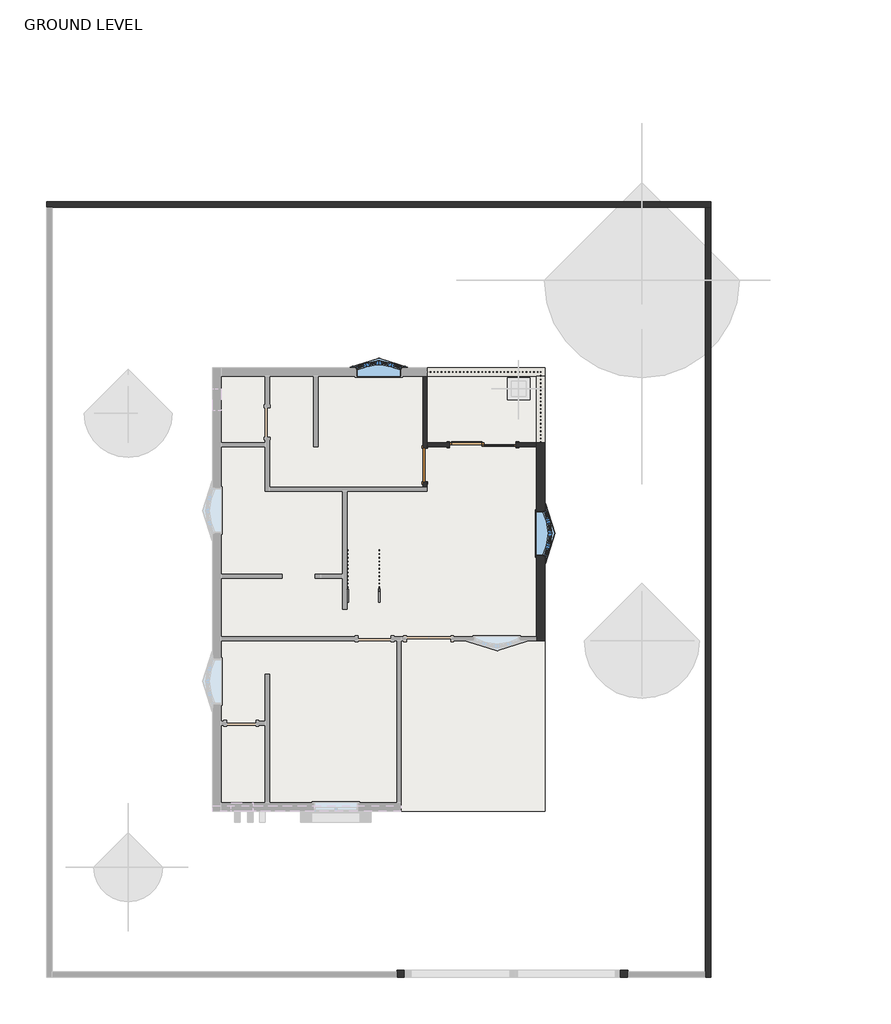
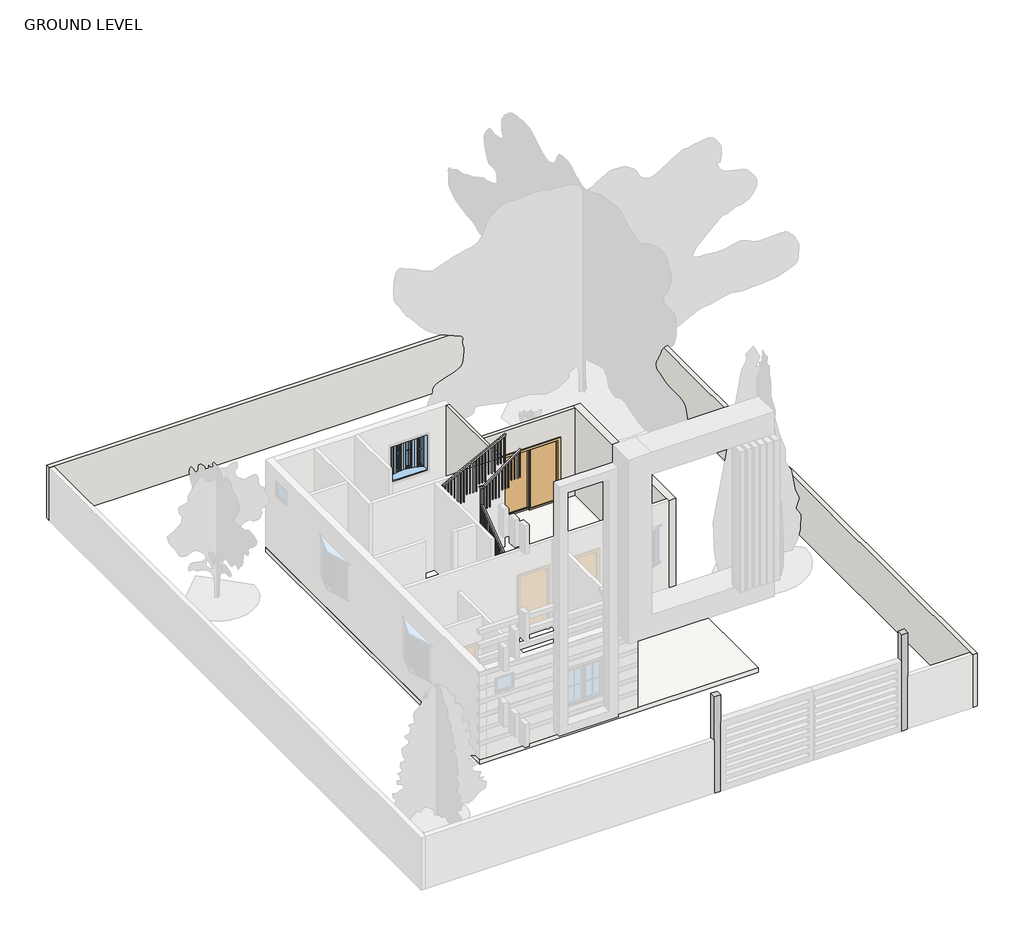
# One storey, part 2 of 3: 7 walls, 2 columns, 2 doors, 2 railings, 2 windows, 1 slab.
"""IFC4 building model written with IfcOpenShell, lengths in millimetres."""

from ifc_helpers import new_model, si_unit, frame, origin, origin_with_axes, place, context, project, spatial, polyline, outline, extrude, faceted_brep, transform, mapped, element, save
from components import door_166d4031, single_flush_3_x7_310a3c6c, window_bow_casement_10_degree_angle_4_x4_fc1e5cf1

model = new_model("IFC4")

# Units and contexts
model_context = context("Model", 3, world=origin())
ifc_project = project(units=[si_unit("LENGTHUNIT", "METRE", prefix="MILLI")], contexts=[model_context])

# Site, building, storey
site = spatial("IfcSite", under=ifc_project)
building = spatial("IfcBuilding", under=site)
storey = spatial("IfcBuildingStorey", under=building, Name="GROUND LEVEL", Elevation=0.0)

# Columns
placement = place(None, origin())
element("IfcColumn", 1, ObjectType="Rectangular Column : 8\"x8\"", at=placement, inside=storey, context=model_context, shape_type="Brep", body=[
    faceted_brep([(-556.7415084, -9926.6064015, -152.4), (-556.7415084, -10129.8064015, -152.4), (-759.9415084, -10129.8064015, -152.4), (-759.9415084, -9977.4064015, -152.4), (-759.9415084, -9926.6064015, -152.4), (-556.7415084, -9926.6064015, 3200.4), (-556.7415084, -10129.8064015, 3200.4), (-759.9415084, -10129.8064015, 3200.4), (-759.9415084, -10129.8064015, 1676.4), (-759.9415084, -9926.6064015, 3200.4)], [[[0, 1, 2, 3, 4]], [[5, 6, 1, 0]], [[6, 7, 8, 2, 1]], [[7, 9, 4, 3, 2, 8]], [[9, 5, 0, 4]], [[5, 9, 7, 6]]]),
])
element("IfcColumn", 2, ObjectType="Rectangular Column : 8\"x8\"", at=placement, inside=storey, context=model_context, shape_type="Brep", body=[
    faceted_brep([(5602.7584916, -9926.6064015, -152.4), (5602.7584916, -9977.4064015, -152.4), (5602.7584916, -10129.8064015, -152.4), (5399.5584916, -10129.8064015, -152.4), (5399.5584916, -9926.6064015, -152.4), (5602.7584916, -9926.6064015, 3200.4), (5602.7584916, -10129.8064015, 3200.4), (5602.7584916, -10129.8064015, 1676.4), (5399.5584916, -10129.8064015, 3200.4), (5399.5584916, -9926.6064015, 3200.4)], [[[0, 1, 2, 3, 4]], [[5, 6, 7, 2, 1, 0]], [[6, 8, 3, 2, 7]], [[8, 9, 4, 3]], [[9, 5, 0, 4]], [[5, 9, 8, 6]]]),
])

# Doors
door_shape = door_166d4031(model_context)
element("IfcDoor", 3, ObjectType="Door-Double-Sliding : 72\" x 84\"", at=placement, inside=storey, context=model_context, shape_type="MappedRepresentation", body=[
    mapped(door_shape, transform((1608.6084916, 4392.6435985, 0.0), x_axis=(1.0, 0.0, 0.0), y_axis=(0.0, 1.0, 0.0), z_axis=(0.0, 0.0, 1.0))),
])
single_flush_3_x7_shape = single_flush_3_x7_310a3c6c(model_context)
element("IfcDoor", 4, ObjectType="Single-Flush : 3'X7'", at=placement, inside=storey, context=model_context, shape_type="MappedRepresentation", body=[
    mapped(single_flush_3_x7_shape, transform((14.7584916, 3967.1935985, 0.0), x_axis=(0.0, -1.0, 0.0), y_axis=(1.0, 0.0, 0.0), z_axis=(0.0, 0.0, 1.0))),
])

# Railings
element("IfcRailing", 5, ObjectType="Handrail - Rectangular", at=placement, inside=storey, context=model_context, shape_type="SolidModel", body=[
    faceted_brep([(-1267.9415084, 195.2935985, 990.6), (-1267.9415084, 195.2935985, 927.1), (-1217.1415084, 195.2935985, 927.1), (-1217.1415084, 195.2935985, 990.6), (-1267.9415084, 2252.6935985, 2533.65), (-1267.9415084, 2303.4935985, 2508.25), (-1217.1415084, 2303.4935985, 2508.25), (-1217.1415084, 2252.6935985, 2533.65), (-1267.9415084, 2252.6935985, 3102.3207921), (-1267.9415084, 2303.4935985, 3051.5207921), (-1217.1415084, 2303.4935985, 3051.5207921), (-1217.1415084, 2252.6935985, 3102.3207921), (-1267.9415084, 2379.6935985, 3102.3207921), (-1267.9415084, 2379.6935985, 3051.5207921), (-1217.1415084, 2328.8935985, 3051.5207921), (-1217.1415084, 2328.8935985, 3102.3207921), (-1140.9415084, 2379.6935985, 3102.3207921), (-1124.6881295, 2379.6935985, 3051.5207921), (-1124.6881295, 2328.8935985, 3051.5207921), (-1140.9415084, 2328.8935985, 3102.3207921), (65.5584916, 2379.6935985, 3962.4), (65.5584916, 2328.8935985, 3962.4), (65.5584916, 2328.8935985, 3900.0134329), (65.5584916, 2379.6935985, 3900.0134329)], [[[0, 1, 2, 3]], [[1, 0, 4, 5]], [[2, 1, 5, 6]], [[3, 2, 6, 7]], [[0, 3, 7, 4]], [[5, 4, 8, 9]], [[6, 5, 9, 10]], [[7, 6, 10, 11]], [[4, 7, 11, 8]], [[9, 8, 12, 13]], [[10, 9, 13, 14]], [[11, 10, 14, 15]], [[8, 11, 15, 12]], [[13, 12, 16, 17]], [[14, 13, 17, 18]], [[15, 14, 18, 19]], [[12, 15, 19, 16]], [[20, 21, 22, 23]], [[17, 16, 20, 23]], [[18, 17, 23, 22]], [[19, 18, 22, 21]], [[16, 19, 21, 20]]]),
    extrude(outline(polyline([(3843.4292745, -13.8165084), (3829.8490764, -32.8665084), (2971.8, -32.8665084), (2971.8, -13.8165084), (3843.4292745, -13.8165084)])), frame((0.0, 2344.7685985, 0.0), z_axis=(0.0, 1.0, 0.0), x_axis=(0.0, 0.0, 1.0)), (0.0, 0.0, 1.0), 19.05),
    extrude(outline(polyline([(3771.0015517, -115.4165084), (3757.4213537, -134.4665084), (2971.8, -134.4665084), (2971.8, -115.4165084), (3771.0015517, -115.4165084)])), frame((0.0, 2344.7685985, 0.0), z_axis=(0.0, 1.0, 0.0), x_axis=(0.0, 0.0, 1.0)), (0.0, 0.0, 1.0), 19.05),
    extrude(outline(polyline([(3698.5738289, -217.0165084), (3684.9936309, -236.0665084), (2971.8, -236.0665084), (2971.8, -217.0165084), (3698.5738289, -217.0165084)])), frame((0.0, 2344.7685985, 0.0), z_axis=(0.0, 1.0, 0.0), x_axis=(0.0, 0.0, 1.0)), (0.0, 0.0, 1.0), 19.05),
    extrude(outline(polyline([(3626.1461062, -318.6165084), (3612.5659081, -337.6665084), (2743.2, -337.6665084), (2743.2, -318.6165084), (3626.1461062, -318.6165084)])), frame((0.0, 2344.7685985, 0.0), z_axis=(0.0, 1.0, 0.0), x_axis=(0.0, 0.0, 1.0)), (0.0, 0.0, 1.0), 19.05),
    extrude(outline(polyline([(3553.7183834, -420.2165084), (3540.1381854, -439.2665084), (2743.2, -439.2665084), (2743.2, -420.2165084), (3553.7183834, -420.2165084)])), frame((0.0, 2344.7685985, 0.0), z_axis=(0.0, 1.0, 0.0), x_axis=(0.0, 0.0, 1.0)), (0.0, 0.0, 1.0), 19.05),
    extrude(outline(polyline([(3481.2906606, -521.8165084), (3467.7104626, -540.8665084), (2743.2, -540.8665084), (2743.2, -521.8165084), (3481.2906606, -521.8165084)])), frame((0.0, 2344.7685985, 0.0), z_axis=(0.0, 1.0, 0.0), x_axis=(0.0, 0.0, 1.0)), (0.0, 0.0, 1.0), 19.05),
    extrude(outline(polyline([(3408.8629378, -623.4165084), (3395.2827398, -642.4665084), (2514.6, -642.4665084), (2514.6, -623.4165084), (3408.8629378, -623.4165084)])), frame((0.0, 2344.7685985, 0.0), z_axis=(0.0, 1.0, 0.0), x_axis=(0.0, 0.0, 1.0)), (0.0, 0.0, 1.0), 19.05),
    extrude(outline(polyline([(3336.4352151, -725.0165084), (3322.855017, -744.0665084), (2514.6, -744.0665084), (2514.6, -725.0165084), (3336.4352151, -725.0165084)])), frame((0.0, 2344.7685985, 0.0), z_axis=(0.0, 1.0, 0.0), x_axis=(0.0, 0.0, 1.0)), (0.0, 0.0, 1.0), 19.05),
    extrude(outline(polyline([(3264.0074923, -826.6165084), (3250.4272943, -845.6665084), (2514.6, -845.6665084), (2514.6, -826.6165084), (3264.0074923, -826.6165084)])), frame((0.0, 2344.7685985, 0.0), z_axis=(0.0, 1.0, 0.0), x_axis=(0.0, 0.0, 1.0)), (0.0, 0.0, 1.0), 19.05),
    extrude(outline(polyline([(3191.5797695, -928.2165084), (3177.9995715, -947.2665084), (2286.0, -947.2665084), (2286.0, -928.2165084), (3191.5797695, -928.2165084)])), frame((0.0, 2344.7685985, 0.0), z_axis=(0.0, 1.0, 0.0), x_axis=(0.0, 0.0, 1.0)), (0.0, 0.0, 1.0), 19.05),
    extrude(outline(polyline([(3119.1520467, -1029.8165084), (3105.5718487, -1048.8665084), (2286.0, -1048.8665084), (2286.0, -1029.8165084), (3119.1520467, -1029.8165084)])), frame((0.0, 2344.7685985, 0.0), z_axis=(0.0, 1.0, 0.0), x_axis=(0.0, 0.0, 1.0)), (0.0, 0.0, 1.0), 19.05),
    extrude(outline(polyline([(3046.724324, -1131.4165084), (3033.144126, -1150.4665084), (2286.0, -1150.4665084), (2286.0, -1131.4165084), (3046.724324, -1131.4165084)])), frame((0.0, 2344.7685985, 0.0), z_axis=(0.0, 1.0, 0.0), x_axis=(0.0, 0.0, 1.0)), (0.0, 0.0, 1.0), 19.05),
    extrude(outline(polyline([(-1233.0165084, 2319.3685985), (-1252.0665084, 2319.3685985), (-1252.0665084, 2338.4185985), (-1233.0165084, 2338.4185985), (-1233.0165084, 2319.3685985)])), frame((0.0, 0.0, 1828.8), z_axis=(0.0, 0.0, 1.0), x_axis=(1.0, 0.0, 0.0)), (0.0, 0.0, 1.0), 1222.7207921),
    extrude(outline(polyline([(2217.7685985, 2443.95625), (2236.8185985, 2458.24375), (2236.8185985, 1600.2), (2217.7685985, 1600.2), (2217.7685985, 2443.95625)])), frame((-1252.0665084, 0.0, 0.0), z_axis=(1.0, 0.0, 0.0), x_axis=(0.0, 1.0, 0.0)), (0.0, 0.0, 1.0), 19.05),
    extrude(outline(polyline([(2116.1685985, 2367.75625), (2135.2185985, 2382.04375), (2135.2185985, 1600.2), (2116.1685985, 1600.2), (2116.1685985, 2367.75625)])), frame((-1252.0665084, 0.0, 0.0), z_axis=(1.0, 0.0, 0.0), x_axis=(0.0, 1.0, 0.0)), (0.0, 0.0, 1.0), 19.05),
    extrude(outline(polyline([(2014.5685985, 2291.55625), (2033.6185985, 2305.84375), (2033.6185985, 1600.2), (2014.5685985, 1600.2), (2014.5685985, 2291.55625)])), frame((-1252.0665084, 0.0, 0.0), z_axis=(1.0, 0.0, 0.0), x_axis=(0.0, 1.0, 0.0)), (0.0, 0.0, 1.0), 19.05),
    extrude(outline(polyline([(1912.9685985, 2215.35625), (1932.0185985, 2229.64375), (1932.0185985, 1371.6), (1912.9685985, 1371.6), (1912.9685985, 2215.35625)])), frame((-1252.0665084, 0.0, 0.0), z_axis=(1.0, 0.0, 0.0), x_axis=(0.0, 1.0, 0.0)), (0.0, 0.0, 1.0), 19.05),
    extrude(outline(polyline([(1811.3685985, 2139.15625), (1830.4185985, 2153.44375), (1830.4185985, 1371.6), (1811.3685985, 1371.6), (1811.3685985, 2139.15625)])), frame((-1252.0665084, 0.0, 0.0), z_axis=(1.0, 0.0, 0.0), x_axis=(0.0, 1.0, 0.0)), (0.0, 0.0, 1.0), 19.05),
    extrude(outline(polyline([(1709.7685985, 2062.95625), (1728.8185985, 2077.24375), (1728.8185985, 1371.6), (1709.7685985, 1371.6), (1709.7685985, 2062.95625)])), frame((-1252.0665084, 0.0, 0.0), z_axis=(1.0, 0.0, 0.0), x_axis=(0.0, 1.0, 0.0)), (0.0, 0.0, 1.0), 19.05),
    extrude(outline(polyline([(1608.1685985, 1986.75625), (1627.2185985, 2001.04375), (1627.2185985, 1143.0), (1608.1685985, 1143.0), (1608.1685985, 1986.75625)])), frame((-1252.0665084, 0.0, 0.0), z_axis=(1.0, 0.0, 0.0), x_axis=(0.0, 1.0, 0.0)), (0.0, 0.0, 1.0), 19.05),
    extrude(outline(polyline([(1506.5685985, 1910.55625), (1525.6185985, 1924.84375), (1525.6185985, 1143.0), (1506.5685985, 1143.0), (1506.5685985, 1910.55625)])), frame((-1252.0665084, 0.0, 0.0), z_axis=(1.0, 0.0, 0.0), x_axis=(0.0, 1.0, 0.0)), (0.0, 0.0, 1.0), 19.05),
    extrude(outline(polyline([(1404.9685985, 1834.35625), (1424.0185985, 1848.64375), (1424.0185985, 1143.0), (1404.9685985, 1143.0), (1404.9685985, 1834.35625)])), frame((-1252.0665084, 0.0, 0.0), z_axis=(1.0, 0.0, 0.0), x_axis=(0.0, 1.0, 0.0)), (0.0, 0.0, 1.0), 19.05),
    extrude(outline(polyline([(1303.3685985, 1758.15625), (1322.4185985, 1772.44375), (1322.4185985, 914.4), (1303.3685985, 914.4), (1303.3685985, 1758.15625)])), frame((-1252.0665084, 0.0, 0.0), z_axis=(1.0, 0.0, 0.0), x_axis=(0.0, 1.0, 0.0)), (0.0, 0.0, 1.0), 19.05),
    extrude(outline(polyline([(1201.7685985, 1681.95625), (1220.8185985, 1696.24375), (1220.8185985, 914.4), (1201.7685985, 914.4), (1201.7685985, 1681.95625)])), frame((-1252.0665084, 0.0, 0.0), z_axis=(1.0, 0.0, 0.0), x_axis=(0.0, 1.0, 0.0)), (0.0, 0.0, 1.0), 19.05),
    extrude(outline(polyline([(1100.1685985, 1605.75625), (1119.2185985, 1620.04375), (1119.2185985, 914.4), (1100.1685985, 914.4), (1100.1685985, 1605.75625)])), frame((-1252.0665084, 0.0, 0.0), z_axis=(1.0, 0.0, 0.0), x_axis=(0.0, 1.0, 0.0)), (0.0, 0.0, 1.0), 19.05),
    extrude(outline(polyline([(998.5685985, 1529.55625), (1017.6185985, 1543.84375), (1017.6185985, 685.8), (998.5685985, 685.8), (998.5685985, 1529.55625)])), frame((-1252.0665084, 0.0, 0.0), z_axis=(1.0, 0.0, 0.0), x_axis=(0.0, 1.0, 0.0)), (0.0, 0.0, 1.0), 19.05),
    extrude(outline(polyline([(896.9685985, 1453.35625), (916.0185985, 1467.64375), (916.0185985, 685.8), (896.9685985, 685.8), (896.9685985, 1453.35625)])), frame((-1252.0665084, 0.0, 0.0), z_axis=(1.0, 0.0, 0.0), x_axis=(0.0, 1.0, 0.0)), (0.0, 0.0, 1.0), 19.05),
    extrude(outline(polyline([(795.3685985, 1377.15625), (814.4185985, 1391.44375), (814.4185985, 685.8), (795.3685985, 685.8), (795.3685985, 1377.15625)])), frame((-1252.0665084, 0.0, 0.0), z_axis=(1.0, 0.0, 0.0), x_axis=(0.0, 1.0, 0.0)), (0.0, 0.0, 1.0), 19.05),
    extrude(outline(polyline([(693.7685985, 1300.95625), (712.8185985, 1315.24375), (712.8185985, 457.2), (693.7685985, 457.2), (693.7685985, 1300.95625)])), frame((-1252.0665084, 0.0, 0.0), z_axis=(1.0, 0.0, 0.0), x_axis=(0.0, 1.0, 0.0)), (0.0, 0.0, 1.0), 19.05),
    extrude(outline(polyline([(592.1685985, 1224.75625), (611.2185985, 1239.04375), (611.2185985, 457.2), (592.1685985, 457.2), (592.1685985, 1224.75625)])), frame((-1252.0665084, 0.0, 0.0), z_axis=(1.0, 0.0, 0.0), x_axis=(0.0, 1.0, 0.0)), (0.0, 0.0, 1.0), 19.05),
    extrude(outline(polyline([(490.5685985, 1148.55625), (509.6185985, 1162.84375), (509.6185985, 457.2), (490.5685985, 457.2), (490.5685985, 1148.55625)])), frame((-1252.0665084, 0.0, 0.0), z_axis=(1.0, 0.0, 0.0), x_axis=(0.0, 1.0, 0.0)), (0.0, 0.0, 1.0), 19.05),
    extrude(outline(polyline([(388.9685985, 1072.35625), (408.0185985, 1086.64375), (408.0185985, 228.6), (388.9685985, 228.6), (388.9685985, 1072.35625)])), frame((-1252.0665084, 0.0, 0.0), z_axis=(1.0, 0.0, 0.0), x_axis=(0.0, 1.0, 0.0)), (0.0, 0.0, 1.0), 19.05),
    extrude(outline(polyline([(287.3685985, 996.15625), (306.4185985, 1010.44375), (306.4185985, 228.6), (287.3685985, 228.6), (287.3685985, 996.15625)])), frame((-1252.0665084, 0.0, 0.0), z_axis=(1.0, 0.0, 0.0), x_axis=(0.0, 1.0, 0.0)), (0.0, 0.0, 1.0), 19.05),
    extrude(outline(polyline([(-1233.0165084, 2344.7685985), (-1252.0665084, 2344.7685985), (-1252.0665084, 2363.8185985), (-1233.0165084, 2363.8185985), (-1233.0165084, 2344.7685985)])), frame((0.0, 0.0, 1828.8), z_axis=(0.0, 0.0, 1.0), x_axis=(1.0, 0.0, 0.0)), (0.0, 0.0, 1.0), 1222.7207921),
    extrude(outline(polyline([(3900.0134329, 65.5584916), (3886.4332349, 46.5084916), (2971.8, 46.5084916), (2971.8, 65.5584916), (3900.0134329, 65.5584916)])), frame((0.0, 2344.7685985, 0.0), z_axis=(0.0, 1.0, 0.0), x_axis=(0.0, 0.0, 1.0)), (0.0, 0.0, 1.0), 19.05),
    extrude(outline(polyline([(195.2935985, 927.1), (214.3435985, 941.3875), (214.3435985, 228.6), (195.2935985, 228.6), (195.2935985, 927.1)])), frame((-1252.0665084, 0.0, 0.0), z_axis=(1.0, 0.0, 0.0), x_axis=(0.0, 1.0, 0.0)), (0.0, 0.0, 1.0), 19.05),
])
element("IfcRailing", 6, ObjectType="Handrail - Rectangular", at=placement, inside=storey, context=model_context, shape_type="SolidModel", body=[
    faceted_brep([(-2131.5415084, 195.2935985, 990.6), (-2131.5415084, 195.2935985, 931.3575287), (-2080.7415084, 195.2935985, 931.3575287), (-2080.7415084, 195.2935985, 990.6), (-2131.5415084, 3116.2935985, 2743.2), (-2131.5415084, 3167.0935985, 2714.4375287), (-2080.7415084, 3167.0935985, 2714.4375287), (-2080.7415084, 3116.2935985, 2743.2), (-2131.5415084, 3116.2935985, 2885.4693642), (-2131.5415084, 3167.0935985, 2834.6693642), (-2080.7415084, 3167.0935985, 2834.6693642), (-2080.7415084, 3116.2935985, 2885.4693642), (-2131.5415084, 3243.2935985, 2885.4693642), (-2131.5415084, 3243.2935985, 2834.6693642), (-2080.7415084, 3192.4935985, 2834.6693642), (-2080.7415084, 3192.4935985, 2885.4693642), (-2004.5415084, 3243.2935985, 2885.4693642), (-1992.1179416, 3243.2935985, 2834.6693642), (-1992.1179416, 3192.4935985, 2834.6693642), (-2004.5415084, 3192.4935985, 2885.4693642), (65.5584916, 3243.2935985, 3962.4), (65.5584916, 3192.4935985, 3962.4), (65.5584916, 3192.4935985, 3905.1368728), (65.5584916, 3243.2935985, 3905.1368728)], [[[0, 1, 2, 3]], [[1, 0, 4, 5]], [[2, 1, 5, 6]], [[3, 2, 6, 7]], [[0, 3, 7, 4]], [[5, 4, 8, 9]], [[6, 5, 9, 10]], [[7, 6, 10, 11]], [[4, 7, 11, 8]], [[9, 8, 12, 13]], [[10, 9, 13, 14]], [[11, 10, 14, 15]], [[8, 11, 15, 12]], [[13, 12, 16, 17]], [[14, 13, 17, 18]], [[15, 14, 18, 19]], [[12, 15, 19, 16]], [[20, 21, 22, 23]], [[17, 16, 20, 23]], [[18, 17, 23, 22]], [[19, 18, 22, 21]], [[16, 19, 21, 20]]]),
    extrude(outline(polyline([(3880.3608612, 17.9334916), (2971.8, 17.9334916), (2971.8, 36.9834916), (3890.2712658, 36.9834916), (3880.3608612, 17.9334916)])), frame((0.0, 3208.3685985, 0.0), z_axis=(0.0, 1.0, 0.0), x_axis=(0.0, 0.0, 1.0)), (0.0, 0.0, 1.0), 19.05),
    extrude(outline(polyline([(3827.5053699, -83.6665084), (2971.8, -83.6665084), (2971.8, -64.6165084), (3837.4157745, -64.6165084), (3827.5053699, -83.6665084)])), frame((0.0, 3208.3685985, 0.0), z_axis=(0.0, 1.0, 0.0), x_axis=(0.0, 0.0, 1.0)), (0.0, 0.0, 1.0), 19.05),
    extrude(outline(polyline([(3774.6498785, -185.2665084), (2971.8, -185.2665084), (2971.8, -166.2165084), (3784.5602832, -166.2165084), (3774.6498785, -185.2665084)])), frame((0.0, 3208.3685985, 0.0), z_axis=(0.0, 1.0, 0.0), x_axis=(0.0, 0.0, 1.0)), (0.0, 0.0, 1.0), 19.05),
    extrude(outline(polyline([(3721.7943872, -286.8665084), (2743.2, -286.8665084), (2743.2, -267.8165084), (3731.7047918, -267.8165084), (3721.7943872, -286.8665084)])), frame((0.0, 3208.3685985, 0.0), z_axis=(0.0, 1.0, 0.0), x_axis=(0.0, 0.0, 1.0)), (0.0, 0.0, 1.0), 19.05),
    extrude(outline(polyline([(3668.9388959, -388.4665084), (2743.2, -388.4665084), (2743.2, -369.4165084), (3678.8493005, -369.4165084), (3668.9388959, -388.4665084)])), frame((0.0, 3208.3685985, 0.0), z_axis=(0.0, 1.0, 0.0), x_axis=(0.0, 0.0, 1.0)), (0.0, 0.0, 1.0), 19.05),
    extrude(outline(polyline([(3616.0834046, -490.0665084), (2743.2, -490.0665084), (2743.2, -471.0165084), (3625.9938092, -471.0165084), (3616.0834046, -490.0665084)])), frame((0.0, 3208.3685985, 0.0), z_axis=(0.0, 1.0, 0.0), x_axis=(0.0, 0.0, 1.0)), (0.0, 0.0, 1.0), 19.05),
    extrude(outline(polyline([(3563.2279132, -591.6665084), (2514.6, -591.6665084), (2514.6, -572.6165084), (3573.1383179, -572.6165084), (3563.2279132, -591.6665084)])), frame((0.0, 3208.3685985, 0.0), z_axis=(0.0, 1.0, 0.0), x_axis=(0.0, 0.0, 1.0)), (0.0, 0.0, 1.0), 19.05),
    extrude(outline(polyline([(3510.3724219, -693.2665084), (2514.6, -693.2665084), (2514.6, -674.2165084), (3520.2828265, -674.2165084), (3510.3724219, -693.2665084)])), frame((0.0, 3208.3685985, 0.0), z_axis=(0.0, 1.0, 0.0), x_axis=(0.0, 0.0, 1.0)), (0.0, 0.0, 1.0), 19.05),
    extrude(outline(polyline([(3457.5169306, -794.8665084), (2514.6, -794.8665084), (2514.6, -775.8165084), (3467.4273352, -775.8165084), (3457.5169306, -794.8665084)])), frame((0.0, 3208.3685985, 0.0), z_axis=(0.0, 1.0, 0.0), x_axis=(0.0, 0.0, 1.0)), (0.0, 0.0, 1.0), 19.05),
    extrude(outline(polyline([(3404.6614392, -896.4665084), (2286.0, -896.4665084), (2286.0, -877.4165084), (3414.5718439, -877.4165084), (3404.6614392, -896.4665084)])), frame((0.0, 3208.3685985, 0.0), z_axis=(0.0, 1.0, 0.0), x_axis=(0.0, 0.0, 1.0)), (0.0, 0.0, 1.0), 19.05),
    extrude(outline(polyline([(3351.8059479, -998.0665084), (2286.0, -998.0665084), (2286.0, -979.0165084), (3361.7163525, -979.0165084), (3351.8059479, -998.0665084)])), frame((0.0, 3208.3685985, 0.0), z_axis=(0.0, 1.0, 0.0), x_axis=(0.0, 0.0, 1.0)), (0.0, 0.0, 1.0), 19.05),
    extrude(outline(polyline([(3298.9504566, -1099.6665084), (2286.0, -1099.6665084), (2286.0, -1080.6165084), (3308.8608612, -1080.6165084), (3298.9504566, -1099.6665084)])), frame((0.0, 3208.3685985, 0.0), z_axis=(0.0, 1.0, 0.0), x_axis=(0.0, 0.0, 1.0)), (0.0, 0.0, 1.0), 19.05),
    extrude(outline(polyline([(3246.0949652, -1201.2665084), (2286.0, -1201.2665084), (2286.0, -1182.2165084), (3256.0053699, -1182.2165084), (3246.0949652, -1201.2665084)])), frame((0.0, 3208.3685985, 0.0), z_axis=(0.0, 1.0, 0.0), x_axis=(0.0, 0.0, 1.0)), (0.0, 0.0, 1.0), 19.05),
    extrude(outline(polyline([(3193.2394739, -1302.8665084), (2057.4, -1302.8665084), (2057.4, -1283.8165084), (3203.1498785, -1283.8165084), (3193.2394739, -1302.8665084)])), frame((0.0, 3208.3685985, 0.0), z_axis=(0.0, 1.0, 0.0), x_axis=(0.0, 0.0, 1.0)), (0.0, 0.0, 1.0), 19.05),
    extrude(outline(polyline([(3140.3839826, -1404.4665084), (2057.4, -1404.4665084), (2057.4, -1385.4165084), (3150.2943872, -1385.4165084), (3140.3839826, -1404.4665084)])), frame((0.0, 3208.3685985, 0.0), z_axis=(0.0, 1.0, 0.0), x_axis=(0.0, 0.0, 1.0)), (0.0, 0.0, 1.0), 19.05),
    extrude(outline(polyline([(3087.5284913, -1506.0665084), (2057.4, -1506.0665084), (2057.4, -1487.0165084), (3097.4388959, -1487.0165084), (3087.5284913, -1506.0665084)])), frame((0.0, 3208.3685985, 0.0), z_axis=(0.0, 1.0, 0.0), x_axis=(0.0, 0.0, 1.0)), (0.0, 0.0, 1.0), 19.05),
    extrude(outline(polyline([(3034.6729999, -1607.6665084), (2057.4, -1607.6665084), (2057.4, -1588.6165084), (3044.5834046, -1588.6165084), (3034.6729999, -1607.6665084)])), frame((0.0, 3208.3685985, 0.0), z_axis=(0.0, 1.0, 0.0), x_axis=(0.0, 0.0, 1.0)), (0.0, 0.0, 1.0), 19.05),
    extrude(outline(polyline([(2981.8175086, -1709.2665084), (2057.4, -1709.2665084), (2057.4, -1690.2165084), (2991.7279132, -1690.2165084), (2981.8175086, -1709.2665084)])), frame((0.0, 3208.3685985, 0.0), z_axis=(0.0, 1.0, 0.0), x_axis=(0.0, 0.0, 1.0)), (0.0, 0.0, 1.0), 19.05),
    extrude(outline(polyline([(2928.9620173, -1810.8665084), (2057.4, -1810.8665084), (2057.4, -1791.8165084), (2938.8724219, -1791.8165084), (2928.9620173, -1810.8665084)])), frame((0.0, 3208.3685985, 0.0), z_axis=(0.0, 1.0, 0.0), x_axis=(0.0, 0.0, 1.0)), (0.0, 0.0, 1.0), 19.05),
    extrude(outline(polyline([(2876.1065259, -1912.4665084), (2057.4, -1912.4665084), (2057.4, -1893.4165084), (2886.0169306, -1893.4165084), (2876.1065259, -1912.4665084)])), frame((0.0, 3208.3685985, 0.0), z_axis=(0.0, 1.0, 0.0), x_axis=(0.0, 0.0, 1.0)), (0.0, 0.0, 1.0), 19.05),
    extrude(outline(polyline([(2823.2510346, -2014.0665084), (2057.4, -2014.0665084), (2057.4, -1995.0165084), (2833.1614392, -1995.0165084), (2823.2510346, -2014.0665084)])), frame((0.0, 3208.3685985, 0.0), z_axis=(0.0, 1.0, 0.0), x_axis=(0.0, 0.0, 1.0)), (0.0, 0.0, 1.0), 19.05),
    extrude(outline(polyline([(-2115.6665084, 3132.1685985), (-2115.6665084, 3151.2185985), (-2096.6165084, 3151.2185985), (-2096.6165084, 3132.1685985), (-2115.6665084, 3132.1685985)])), frame((0.0, 0.0, 1828.8), z_axis=(0.0, 0.0, 1.0), x_axis=(1.0, 0.0, 0.0)), (0.0, 0.0, 1.0), 1005.8693642),
    extrude(outline(polyline([(3049.6185985, 2643.9525287), (3049.6185985, 1828.8), (3030.5685985, 1828.8), (3030.5685985, 2632.5225287), (3049.6185985, 2643.9525287)])), frame((-2115.6665084, 0.0, 0.0), z_axis=(1.0, 0.0, 0.0), x_axis=(0.0, 1.0, 0.0)), (0.0, 0.0, 1.0), 19.05),
    extrude(outline(polyline([(2948.0185985, 2582.9925287), (2948.0185985, 1828.8), (2928.9685985, 1828.8), (2928.9685985, 2571.5625287), (2948.0185985, 2582.9925287)])), frame((-2115.6665084, 0.0, 0.0), z_axis=(1.0, 0.0, 0.0), x_axis=(0.0, 1.0, 0.0)), (0.0, 0.0, 1.0), 19.05),
    extrude(outline(polyline([(2846.4185985, 2522.0325287), (2846.4185985, 1828.8), (2827.3685985, 1828.8), (2827.3685985, 2510.6025287), (2846.4185985, 2522.0325287)])), frame((-2115.6665084, 0.0, 0.0), z_axis=(1.0, 0.0, 0.0), x_axis=(0.0, 1.0, 0.0)), (0.0, 0.0, 1.0), 19.05),
    extrude(outline(polyline([(2744.8185985, 2461.0725287), (2744.8185985, 1828.8), (2725.7685985, 1828.8), (2725.7685985, 2449.6425287), (2744.8185985, 2461.0725287)])), frame((-2115.6665084, 0.0, 0.0), z_axis=(1.0, 0.0, 0.0), x_axis=(0.0, 1.0, 0.0)), (0.0, 0.0, 1.0), 19.05),
    extrude(outline(polyline([(2643.2185985, 2400.1125287), (2643.2185985, 1828.8), (2624.1685985, 1828.8), (2624.1685985, 2388.6825287), (2643.2185985, 2400.1125287)])), frame((-2115.6665084, 0.0, 0.0), z_axis=(1.0, 0.0, 0.0), x_axis=(0.0, 1.0, 0.0)), (0.0, 0.0, 1.0), 19.05),
    extrude(outline(polyline([(2541.6185985, 2339.1525287), (2541.6185985, 1828.8), (2522.5685985, 1828.8), (2522.5685985, 2327.7225287), (2541.6185985, 2339.1525287)])), frame((-2115.6665084, 0.0, 0.0), z_axis=(1.0, 0.0, 0.0), x_axis=(0.0, 1.0, 0.0)), (0.0, 0.0, 1.0), 19.05),
    extrude(outline(polyline([(2440.0185985, 2278.1925287), (2440.0185985, 1828.8), (2420.9685985, 1828.8), (2420.9685985, 2266.7625287), (2440.0185985, 2278.1925287)])), frame((-2115.6665084, 0.0, 0.0), z_axis=(1.0, 0.0, 0.0), x_axis=(0.0, 1.0, 0.0)), (0.0, 0.0, 1.0), 19.05),
    extrude(outline(polyline([(2338.4185985, 2217.2325287), (2338.4185985, 1828.8), (2319.3685985, 1828.8), (2319.3685985, 2205.8025287), (2338.4185985, 2217.2325287)])), frame((-2115.6665084, 0.0, 0.0), z_axis=(1.0, 0.0, 0.0), x_axis=(0.0, 1.0, 0.0)), (0.0, 0.0, 1.0), 19.05),
    extrude(outline(polyline([(2236.8185985, 2156.2725287), (2236.8185985, 1600.2), (2217.7685985, 1600.2), (2217.7685985, 2144.8425287), (2236.8185985, 2156.2725287)])), frame((-2115.6665084, 0.0, 0.0), z_axis=(1.0, 0.0, 0.0), x_axis=(0.0, 1.0, 0.0)), (0.0, 0.0, 1.0), 19.05),
    extrude(outline(polyline([(2135.2185985, 2095.3125287), (2135.2185985, 1600.2), (2116.1685985, 1600.2), (2116.1685985, 2083.8825287), (2135.2185985, 2095.3125287)])), frame((-2115.6665084, 0.0, 0.0), z_axis=(1.0, 0.0, 0.0), x_axis=(0.0, 1.0, 0.0)), (0.0, 0.0, 1.0), 19.05),
    extrude(outline(polyline([(2033.6185985, 2034.3525287), (2033.6185985, 1600.2), (2014.5685985, 1600.2), (2014.5685985, 2022.9225287), (2033.6185985, 2034.3525287)])), frame((-2115.6665084, 0.0, 0.0), z_axis=(1.0, 0.0, 0.0), x_axis=(0.0, 1.0, 0.0)), (0.0, 0.0, 1.0), 19.05),
    extrude(outline(polyline([(1932.0185985, 1973.3925287), (1932.0185985, 1371.6), (1912.9685985, 1371.6), (1912.9685985, 1961.9625287), (1932.0185985, 1973.3925287)])), frame((-2115.6665084, 0.0, 0.0), z_axis=(1.0, 0.0, 0.0), x_axis=(0.0, 1.0, 0.0)), (0.0, 0.0, 1.0), 19.05),
    extrude(outline(polyline([(1830.4185985, 1912.4325287), (1830.4185985, 1371.6), (1811.3685985, 1371.6), (1811.3685985, 1901.0025287), (1830.4185985, 1912.4325287)])), frame((-2115.6665084, 0.0, 0.0), z_axis=(1.0, 0.0, 0.0), x_axis=(0.0, 1.0, 0.0)), (0.0, 0.0, 1.0), 19.05),
    extrude(outline(polyline([(1728.8185985, 1851.4725287), (1728.8185985, 1371.6), (1709.7685985, 1371.6), (1709.7685985, 1840.0425287), (1728.8185985, 1851.4725287)])), frame((-2115.6665084, 0.0, 0.0), z_axis=(1.0, 0.0, 0.0), x_axis=(0.0, 1.0, 0.0)), (0.0, 0.0, 1.0), 19.05),
    extrude(outline(polyline([(1627.2185985, 1790.5125287), (1627.2185985, 1143.0), (1608.1685985, 1143.0), (1608.1685985, 1779.0825287), (1627.2185985, 1790.5125287)])), frame((-2115.6665084, 0.0, 0.0), z_axis=(1.0, 0.0, 0.0), x_axis=(0.0, 1.0, 0.0)), (0.0, 0.0, 1.0), 19.05),
    extrude(outline(polyline([(1525.6185985, 1729.5525287), (1525.6185985, 1143.0), (1506.5685985, 1143.0), (1506.5685985, 1718.1225287), (1525.6185985, 1729.5525287)])), frame((-2115.6665084, 0.0, 0.0), z_axis=(1.0, 0.0, 0.0), x_axis=(0.0, 1.0, 0.0)), (0.0, 0.0, 1.0), 19.05),
    extrude(outline(polyline([(1424.0185985, 1668.5925287), (1424.0185985, 1143.0), (1404.9685985, 1143.0), (1404.9685985, 1657.1625287), (1424.0185985, 1668.5925287)])), frame((-2115.6665084, 0.0, 0.0), z_axis=(1.0, 0.0, 0.0), x_axis=(0.0, 1.0, 0.0)), (0.0, 0.0, 1.0), 19.05),
    extrude(outline(polyline([(1322.4185985, 1607.6325287), (1322.4185985, 914.4), (1303.3685985, 914.4), (1303.3685985, 1596.2025287), (1322.4185985, 1607.6325287)])), frame((-2115.6665084, 0.0, 0.0), z_axis=(1.0, 0.0, 0.0), x_axis=(0.0, 1.0, 0.0)), (0.0, 0.0, 1.0), 19.05),
    extrude(outline(polyline([(1220.8185985, 1546.6725287), (1220.8185985, 914.4), (1201.7685985, 914.4), (1201.7685985, 1535.2425287), (1220.8185985, 1546.6725287)])), frame((-2115.6665084, 0.0, 0.0), z_axis=(1.0, 0.0, 0.0), x_axis=(0.0, 1.0, 0.0)), (0.0, 0.0, 1.0), 19.05),
    extrude(outline(polyline([(1119.2185985, 1485.7125287), (1119.2185985, 914.4), (1100.1685985, 914.4), (1100.1685985, 1474.2825287), (1119.2185985, 1485.7125287)])), frame((-2115.6665084, 0.0, 0.0), z_axis=(1.0, 0.0, 0.0), x_axis=(0.0, 1.0, 0.0)), (0.0, 0.0, 1.0), 19.05),
    extrude(outline(polyline([(1017.6185985, 1424.7525287), (1017.6185985, 685.8), (998.5685985, 685.8), (998.5685985, 1413.3225287), (1017.6185985, 1424.7525287)])), frame((-2115.6665084, 0.0, 0.0), z_axis=(1.0, 0.0, 0.0), x_axis=(0.0, 1.0, 0.0)), (0.0, 0.0, 1.0), 19.05),
    extrude(outline(polyline([(916.0185985, 1363.7925287), (916.0185985, 685.8), (896.9685985, 685.8), (896.9685985, 1352.3625287), (916.0185985, 1363.7925287)])), frame((-2115.6665084, 0.0, 0.0), z_axis=(1.0, 0.0, 0.0), x_axis=(0.0, 1.0, 0.0)), (0.0, 0.0, 1.0), 19.05),
    extrude(outline(polyline([(814.4185985, 1302.8325287), (814.4185985, 685.8), (795.3685985, 685.8), (795.3685985, 1291.4025287), (814.4185985, 1302.8325287)])), frame((-2115.6665084, 0.0, 0.0), z_axis=(1.0, 0.0, 0.0), x_axis=(0.0, 1.0, 0.0)), (0.0, 0.0, 1.0), 19.05),
    extrude(outline(polyline([(712.8185985, 1241.8725287), (712.8185985, 457.2), (693.7685985, 457.2), (693.7685985, 1230.4425287), (712.8185985, 1241.8725287)])), frame((-2115.6665084, 0.0, 0.0), z_axis=(1.0, 0.0, 0.0), x_axis=(0.0, 1.0, 0.0)), (0.0, 0.0, 1.0), 19.05),
    extrude(outline(polyline([(611.2185985, 1180.9125287), (611.2185985, 457.2), (592.1685985, 457.2), (592.1685985, 1169.4825287), (611.2185985, 1180.9125287)])), frame((-2115.6665084, 0.0, 0.0), z_axis=(1.0, 0.0, 0.0), x_axis=(0.0, 1.0, 0.0)), (0.0, 0.0, 1.0), 19.05),
    extrude(outline(polyline([(509.6185985, 1119.9525287), (509.6185985, 457.2), (490.5685985, 457.2), (490.5685985, 1108.5225287), (509.6185985, 1119.9525287)])), frame((-2115.6665084, 0.0, 0.0), z_axis=(1.0, 0.0, 0.0), x_axis=(0.0, 1.0, 0.0)), (0.0, 0.0, 1.0), 19.05),
    extrude(outline(polyline([(408.0185985, 1058.9925287), (408.0185985, 228.6), (388.9685985, 228.6), (388.9685985, 1047.5625287), (408.0185985, 1058.9925287)])), frame((-2115.6665084, 0.0, 0.0), z_axis=(1.0, 0.0, 0.0), x_axis=(0.0, 1.0, 0.0)), (0.0, 0.0, 1.0), 19.05),
    extrude(outline(polyline([(306.4185985, 998.0325287), (306.4185985, 228.6), (287.3685985, 228.6), (287.3685985, 986.6025287), (306.4185985, 998.0325287)])), frame((-2115.6665084, 0.0, 0.0), z_axis=(1.0, 0.0, 0.0), x_axis=(0.0, 1.0, 0.0)), (0.0, 0.0, 1.0), 19.05),
    extrude(outline(polyline([(-2115.6665084, 3208.3685985), (-2115.6665084, 3227.4185985), (-2096.6165084, 3227.4185985), (-2096.6165084, 3208.3685985), (-2115.6665084, 3208.3685985)])), frame((0.0, 0.0, 1828.8), z_axis=(0.0, 0.0, 1.0), x_axis=(1.0, 0.0, 0.0)), (0.0, 0.0, 1.0), 1005.8693642),
    extrude(outline(polyline([(3895.2264681, 46.5084916), (2971.8, 46.5084916), (2971.8, 65.5584916), (3905.1368728, 65.5584916), (3895.2264681, 46.5084916)])), frame((0.0, 3208.3685985, 0.0), z_axis=(0.0, 1.0, 0.0), x_axis=(0.0, 0.0, 1.0)), (0.0, 0.0, 1.0), 19.05),
    extrude(outline(polyline([(214.3435985, 942.7875287), (214.3435985, 228.6), (195.2935985, 228.6), (195.2935985, 931.3575287), (214.3435985, 942.7875287)])), frame((-2115.6665084, 0.0, 0.0), z_axis=(1.0, 0.0, 0.0), x_axis=(0.0, 1.0, 0.0)), (0.0, 0.0, 1.0), 19.05),
])

# Slab
element("IfcSlab", 7, ObjectType="6\"", at=placement, inside=storey, context=model_context, shape_type="SweptSolid", body=[
    extrude(outline(polyline([(3316.7584916, 6634.1935985), (3316.7584916, -5557.8064015), (-5827.2415084, -5557.8064015), (-5827.2415084, 6634.1935985), (3316.7584916, 6634.1935985)])), frame((0.0, 0.0, -152.4), z_axis=(0.0, 0.0, 1.0), x_axis=(1.0, 0.0, 0.0)), (0.0, 0.0, 1.0), 152.4),
])

# Walls
element("IfcWall", 8, ObjectType="4\"", at=placement, inside=storey, context=model_context, shape_type="Brep", body=[
    faceted_brep([(-36.0415084, 3509.9935985, 2133.6), (-36.0415084, 3509.9935985, 0.0), (-36.0415084, 3357.5935985, 0.0), (-36.0415084, 3357.5935985, 3048.0), (-36.0415084, 6405.5935985, 3048.0), (-36.0415084, 6405.5935985, 0.0), (-36.0415084, 4424.3935985, 0.0), (-36.0415084, 4424.3935985, 2133.6), (65.5584916, 3357.5935985, 0.0), (65.5584916, 3509.9935985, 0.0), (65.5584916, 3509.9935985, 2133.6), (65.5584916, 4424.3935985, 2133.6), (65.5584916, 4424.3935985, 0.0), (65.5584916, 4462.4935985, 0.0), (65.5584916, 4576.7935985, 0.0), (65.5584916, 6405.5935985, 0.0), (65.5584916, 6405.5935985, 3048.0), (65.5584916, 4576.7935985, 3048.0), (65.5584916, 4462.4935985, 3048.0), (65.5584916, 3357.5935985, 3048.0)], [[[0, 1, 2, 3, 4, 5, 6, 7]], [[8, 9, 10, 11, 12, 13, 14, 15, 16, 17, 18, 19]], [[6, 5, 15, 14, 13, 12]], [[2, 1, 9, 8]], [[4, 3, 19, 18, 17, 16]], [[3, 2, 8, 19]], [[10, 9, 1, 0]], [[11, 10, 0, 7]], [[12, 11, 7, 6]], [[4, 16, 15, 5]]]),
])
element("IfcWall", 9, ObjectType="4.5\"", at=placement, inside=storey, context=model_context, shape_type="SweptSolid", body=[
    extrude(outline(polyline([(2133.6, 2523.0084916), (0.0, 2523.0084916), (0.0, 3088.1584916), (3048.0, 3088.1584916), (3048.0, 65.5584916), (0.0, 65.5584916), (0.0, 694.2084916), (2133.6, 694.2084916), (2133.6, 2523.0084916)])), frame((0.0, 4462.4935985, 0.0), z_axis=(0.0, 1.0, 0.0), x_axis=(0.0, 0.0, 1.0)), (0.0, 0.0, 1.0), 114.3),
])
element("IfcWall", 10, ObjectType="6\"", at=placement, inside=storey, context=model_context, shape_type="Brep", body=[
    faceted_brep([(7888.7584916, 11206.1935985, -152.4), (-10399.2415084, 11206.1935985, -152.4), (-10399.2415084, 11206.1935985, 1676.4), (7888.7584916, 11206.1935985, 1676.4), (7888.7584916, 11053.7935985, -152.4), (7888.7584916, 11053.7935985, 1676.4), (7736.3584916, 11053.7935985, 1676.4), (-10246.8415084, 11053.7935985, 1676.4), (-10399.2415084, 11053.7935985, 1676.4), (-10399.2415084, 11053.7935985, -152.4), (-10246.8415084, 11053.7935985, -152.4), (7736.3584916, 11053.7935985, -152.4)], [[[0, 1, 2, 3]], [[4, 5, 6, 7, 8, 9, 10, 11]], [[1, 0, 4, 11, 10, 9]], [[3, 2, 8, 7, 6, 5]], [[2, 1, 9, 8]], [[0, 3, 5, 4]]]),
])
element("IfcWall", 11, ObjectType="6\"", at=placement, inside=storey, context=model_context, shape_type="Brep", body=[
    faceted_brep([(7888.7584916, -10129.8064015, -152.4), (7888.7584916, 11053.7935985, -152.4), (7888.7584916, 11053.7935985, 1676.4), (7888.7584916, -10129.8064015, 1676.4), (7736.3584916, -10129.8064015, -152.4), (7736.3584916, -10129.8064015, 1676.4), (7736.3584916, -9977.4064015, 1676.4), (7736.3584916, 11053.7935985, 1676.4), (7736.3584916, 11053.7935985, -152.4), (7736.3584916, -9977.4064015, -152.4)], [[[0, 1, 2, 3]], [[4, 5, 6, 7, 8, 9]], [[1, 0, 4, 9, 8]], [[3, 2, 7, 6, 5]], [[2, 1, 8, 7]], [[0, 3, 5, 4]]]),
])
element("IfcWall", 12, ObjectType="9\"", at=placement, inside=storey, context=model_context, shape_type="Brep", body=[
    faceted_brep([(3316.7584916, -871.5064015, 0.0), (3316.7584916, 4576.7935985, 0.0), (3316.7584916, 4576.7935985, 609.6), (3316.7584916, 4576.7935985, 3048.0), (3316.7584916, -871.5064015, 3048.0), (3316.7584916, 1447.7534915, 1879.6), (3316.7584916, 2714.7337055, 1879.6), (3316.7584916, 2714.7337055, 609.6), (3316.7584916, 1447.7534915, 609.6), (3088.1584916, -871.5064015, 0.0), (3088.1584916, -871.5064015, 3048.0), (3088.1584916, -757.2064015, 3048.0), (3088.1584916, 4462.4935985, 3048.0), (3088.1584916, 4576.7935985, 3048.0), (3088.1584916, 4576.7935985, 609.6), (3088.1584916, 4576.7935985, 0.0), (3088.1584916, 4462.4935985, 0.0), (3088.1584916, -757.2064015, 0.0), (3088.1584916, 2690.8435985, 1879.6), (3088.1584916, 1471.6435985, 1879.6), (3088.1584916, 1471.6435985, 609.6), (3088.1584916, 2690.8435985, 609.6), (3251.1209621, 2690.8435985, 1879.6), (3251.1209621, 1471.6435985, 1879.6), (3251.1209621, 2690.8435985, 609.6), (3251.1209621, 1471.6435985, 609.6)], [[[0, 1, 2, 3, 4], [5, 6, 7, 8]], [[9, 10, 11, 12, 13, 14, 15, 16, 17], [18, 19, 20, 21]], [[1, 0, 9, 17, 16, 15]], [[3, 2, 1, 15, 14, 13]], [[4, 3, 13, 12, 11, 10]], [[0, 4, 10, 9]], [[22, 6, 5, 23, 19, 18]], [[24, 21, 20, 25, 8, 7]], [[22, 18, 21, 24]], [[19, 23, 25, 20]], [[23, 5, 8, 25]], [[6, 22, 24, 7]]]),
])
element("IfcWall", 13, ObjectType="9\"", at=placement, inside=storey, context=model_context, shape_type="Brep", body=[
    faceted_brep([(65.5584916, 6405.5935985, 0.0), (3088.1584916, 6405.5935985, 0.0), (3316.7584916, 6405.5935985, 0.0), (3316.7584916, 6405.5935985, 609.6), (3088.1584916, 6405.5935985, 609.6), (65.5584916, 6405.5935985, 609.6), (65.5584916, 6634.1935985, 0.0), (65.5584916, 6634.1935985, 609.6), (3316.7584916, 6634.1935985, 609.6), (3316.7584916, 6634.1935985, 0.0)], [[[0, 1, 2, 3, 4, 5]], [[6, 7, 8, 9]], [[2, 1, 0, 6, 9]], [[5, 4, 3, 8, 7]], [[0, 5, 7, 6]], [[3, 2, 9, 8]]]),
])
element("IfcWall", 14, ObjectType="9\"", at=placement, inside=storey, context=model_context, shape_type="SweptSolid", body=[
    extrude(outline(polyline([(3088.1584916, 4576.7935985), (3088.1584916, 6405.5935985), (3316.7584916, 6405.5935985), (3316.7584916, 4576.7935985), (3088.1584916, 4576.7935985)])), origin_with_axes(), (0.0, 0.0, 1.0), 609.6),
])

# Windows
window_bow_casement_10_degree_angle_4_x4_shape = window_bow_casement_10_degree_angle_4_x4_fc1e5cf1(model_context)
element("IfcWindow", 15, ObjectType="Window-Bow-Casement-10_Degree_Angle : 4'X4'", at=placement, inside=storey, context=model_context, shape_type="MappedRepresentation", body=[
    mapped(window_bow_casement_10_degree_angle_4_x4_shape, transform((-1255.2415084, 6519.8935985, 384.1323709), x_axis=(1.0, 0.0, 0.0), y_axis=(0.0, 1.0, 0.0), z_axis=(0.0, 0.0, 1.0))),
])
element("IfcWindow", 16, ObjectType="Window-Bow-Casement-10_Degree_Angle : 4'X4'", at=placement, inside=storey, context=model_context, shape_type="MappedRepresentation", body=[
    mapped(window_bow_casement_10_degree_angle_4_x4_shape, transform((3202.4584916, 2081.2435985, 0.0), x_axis=(0.0, -1.0, 0.0), y_axis=(1.0, 0.0, 0.0), z_axis=(0.0, 0.0, 1.0))),
])

save(model, "model.ifc")

# Revit data of these elements
# Type "Rectangular Column : 8\"x8\""
#   Assembly Code = "B1010200"
#   Depth = 0' - 8"
#   Offset Base = 0' - 0"
#   Offset Top = 0' - 0"
#   Width = 0' - 8"
#   Material = none
# Type "Door-Double-Sliding : 72\" x 84\""
#   Type Mark = "12"
#   Construction Type Id = "opn-d45"
#   Assembly Code = "C1020"
#   Analytic Construction = "Wood frame, double glass door "
#   Thickness = 0' - 2"
#   Thermal Resistance (R) = 1.8150 (h·ft²·°F)/BTU
#   Heat Transfer Coefficient (U) = 0.5510 BTU/(h·ft²·°F)
#   Height = 7' - 0"
#   Rail Width = 0' - 2"
#   Stiles = 0' - 2"
#   Trim Projection Ext = 0' - 1"
#   Trim Projection Int = 0' - 1"
#   Trim Width = 0' - 3"
#   Width = 6' - 0"
#   Define Thermal Properties by = 1
#   Glazing = Glass
#   Panel Material = Wood - Birch - Solid Stained Light Low Gloss
#   Trim Material = Paint - Sienna
#   Visual Light Transmittance = 0
#   Solar Heat Gain Coefficient = 0
#   Function = (empty or 0)
#   Wall Closure = (empty or 0)
# Type "Single-Flush : 3'X7'"
#   Type Mark = "8"
#   Construction Type Id = "MDOOR"
#   Assembly Code = "C1020"
#   Analytic Construction = "Metal"
#   Thickness = 0' - 2"
#   Heat Transfer Coefficient (U) = 0.651978 BTU/(h·ft²·°F)
#   Height = 7' - 0"
#   Trim Projection Ext = 0' - 1"
#   Trim Projection Int = 0' - 1"
#   Trim Width = 0' - 3"
#   Width = 3' - 0"
#   Define Thermal Properties by = 1
#   Door Material = Door - Panel
#   Frame Material = Door - Frame
#   Visual Light Transmittance = 0
#   Solar Heat Gain Coefficient = 0
#   Function = (empty or 0)
#   Wall Closure = (empty or 0)
# Type "Handrail - Rectangular"
#   Assembly Code = "C2010400"
#   built-in parameter 1008612 = 0.0416667 (stored number, unit not read)
#   built-in parameter 1008611 = 0.0416667 (stored number, unit not read)
#   built-in parameter 1008609 = 0.333333 (stored number, unit not read)
#   built-in parameter 1008604 = 0.166667 (stored number, unit not read)
#   built-in parameter 1008603 = 0.166667 (stored number, unit not read)
#   Railing Height = 2' - 6"
#   built-in parameter 1008630 = 2
#   built-in parameter 1008610 = 2
#   built-in parameter 1008618 = Baluster - Square : 3/4"
# Type "6\""
#   Assembly Code = "B1010"
#   Function = 0
#   Layers, outside or top first: 0' - 6" no material (function 1)
# Type "4\""
#   Assembly Code = "B2010"
#   Layers, outside or top first: 0' - 4" no material (function 1)
# Type "4.5\""
#   Assembly Code = "B2010"
#   Layers, outside or top first: 0' - 4 1/2" no material (function 1)
# Type "6\""
#   Assembly Code = "B2010"
#   Layers, outside or top first: 0' - 6" "6\" wall" (function 1)
# Type "9\""
#   Assembly Code = "B2010"
#   Layers, outside or top first: 0' - 9" "wood" (function 1)
# Type "Window-Bow-Casement-10_Degree_Angle : 4'X4'"
#   Type Mark = "27"
#   Fire Rating = "0.5h"
#   Assembly Code = "B2020100"
#   Analytic Construction = "Double glazing - domestic"
#   Width = 4' - 0"
#   Visual Light Transmittance = 0.81
#   Thermal Resistance (R) = 1.8146 (h·ft²·°F)/BTU
#   Solar Heat Gain Coefficient = 0.76
#   Rough Width = 4' - 0 1/2"
#   Rough Height = 4' - 0 1/2"
#   Radius 3 = 4' - 11.49333"
#   Radius 2 = 4' - 10.49333"
#   Radius 1 = 4' - 8.49333"
#   Length 7 = 4' - 9.19062"
#   Length 6 = 0' - 1.41593"
#   Length 5 = 1' - 1.00986"
#   Length 2 = 0' - 2.58415"
#   Depth 2 = 0' - 6.3557"
#   Length 4 = 0' - 1.03923"
#   Length 3 = 0' - 0.32476"
#   Length 1 = 0' - 10.27567"
#   Wall Thickness [instance default] = 0' - 6"
#   Trim Width = 4' - 4.64952"
#   Trim Height = 4' - 0"
#   Height 1 = 4' - 2"
#   Height = 4' - 0"
#   Heat Transfer Coefficient (U) = 0.5511 BTU/(h·ft²·°F)
#   Depth 1 = 0' - 5.29439"
#   Default Sill Height = 2' - 0"
#   Angle 2 = 15.00°
#   Angle 1 = 10.00°
#   Angle = 20.00°
#   Muntin Visibility = yes
#   Interior Trim Visibility [instance default] = yes
#   Exterior Trim Visibility [instance default] = yes
#   Muntin Pattern = Muntin Pattern_2x2 : Muntin Pattern_2x2
#   Interior Trim Material = Wood - Stained
#   Exterior Trim Material = Clad - White
#   Interior Trim = Trim-Window-Interior-Flat : Picture Frame
#   Interior Frame Material = Wood - Stained
#   Glass Panel Material = Glass
#   Exterior Frame Material = Clad - White
#   Wall Closure = (empty or 0)
# Elements 1, 2 (IfcColumn, "Rectangular Column : 8\"x8\"")
#   Phase Created = New Construction
#   Materials on its faces: "6\" wall"
# Element 3 (IfcDoor, "Door-Double-Sliding : 72\" x 84\"")
#   Phase Created = New Construction
#   Materials on its faces: "Paint - Sienna", "Wood - Birch - Solid Stained Light Low Gloss", "Glass"
# Element 4 (IfcDoor, "Single-Flush : 3'X7'")
#   Phase Created = New Construction
#   Materials on its faces: "Door - Frame", "Door - Panel"
# Elements 5, 6 (IfcRailing, "Handrail - Rectangular")
#   Phase Created = New Construction
# Element 7 (IfcSlab, "6\"")
#   Height Offset From Level = 0' - 0"
#   Phase Created = New Construction
#   Materials on its faces: "Default Floor"
# Element 8 (IfcWall, "4\"")
#   Top Offset = -0' - 6"
#   Base Offset = 0' - 0"
#   wall height = 10' - 0"
#   Phase Created = New Construction
#   Base Constraint = GROUND LEVEL
#   Top Constraint = FIRST FLOOR
#   Materials on its faces: "Default Wall", "wall 1"
# Element 9 (IfcWall, "4.5\"")
#   Top Offset = -0' - 6"
#   Base Offset = 0' - 0"
#   wall height = 10' - 0"
#   Phase Created = New Construction
#   Base Constraint = GROUND LEVEL
#   Top Constraint = FIRST FLOOR
#   Materials on its faces: "Default Wall", "wall 1"
# Elements 10, 11 (IfcWall, "6\"")
#   built-in parameter 1001111 = -0' - 6"
#   Top Offset = -0' - 6"
#   Base Offset = -0' - 6"
#   Unconnected Height = 6' - 0"
#   wall height = 6' - 0"
#   Phase Created = New Construction
#   Base Constraint = GROUND LEVEL
#   Materials on its faces: "6\" wall"
# Element 12 (IfcWall, "9\"")
#   Top Offset = -0' - 6"
#   Base Offset = 0' - 0"
#   wall height = 10' - 0"
#   Phase Created = New Construction
#   Base Constraint = GROUND LEVEL
#   Top Constraint = FIRST FLOOR
#   Materials on its faces: "wood", "6\" wall", "wall 1", "Default Wall"
# Elements 13, 14 (IfcWall, "9\"")
#   Top Offset = -0' - 6"
#   Base Offset = 0' - 0"
#   Unconnected Height = 2' - 0"
#   wall height = 2' - 0"
#   Phase Created = New Construction
#   Base Constraint = GROUND LEVEL
#   Materials on its faces: "wood", "wall 1"
# Element 15 (IfcWindow, "Window-Bow-Casement-10_Degree_Angle : 4'X4'")
#   Mark = "4"
#   Phase Created = New Construction
#   Materials on its faces: "Wood - Stained", "Clad - White", "Glass"
# Element 16 (IfcWindow, "Window-Bow-Casement-10_Degree_Angle : 4'X4'")
#   Mark = "15"
#   Interior Trim Visibility = yes
#   Exterior Trim Visibility = yes
#   Phase Created = New Construction
#   Materials on its faces: "Wood - Stained", "Clad - White", "Glass"
# Materials
#   "Glass": class "Glass", colour RGB 0 128 192, transparency 0.75, Description = "Soda Lime Glass", Cost = 0
#   "Wood - Birch - Solid Stained Light Low Gloss": class "Wood", colour RGB 210 159 95, transparency 0, Cost = 0
#   "Paint - Sienna": colour RGB 118 70 51, transparency 0, Cost = 0
#   "Door - Panel": class "Wood", colour RGB 210 159 95, transparency 0, Cost = 0
#   "Door - Frame": colour RGB 118 70 51, transparency 0, Cost = 0
#   "6\" wall": class "Generic", colour RGB 177 162 144, transparency 0, Cost = 0
#   "wood": class "Generic", colour RGB 188 176 153, transparency 0, Cost = 0
#   "Wood - Stained": class "Wood", colour RGB 224 178 126, transparency 0, Cost = 0
#   "Clad - White": class "Wood", colour RGB 242 242 238, transparency 0, Cost = 0
#   "Default Floor": colour RGB 128 128 128, transparency 0, Cost = 0
#   "Default Wall": colour RGB 128 128 128, transparency 0, Cost = 0
#   "wall 1": class "Generic", colour RGB 67 39 34, transparency 0, Cost = 0
